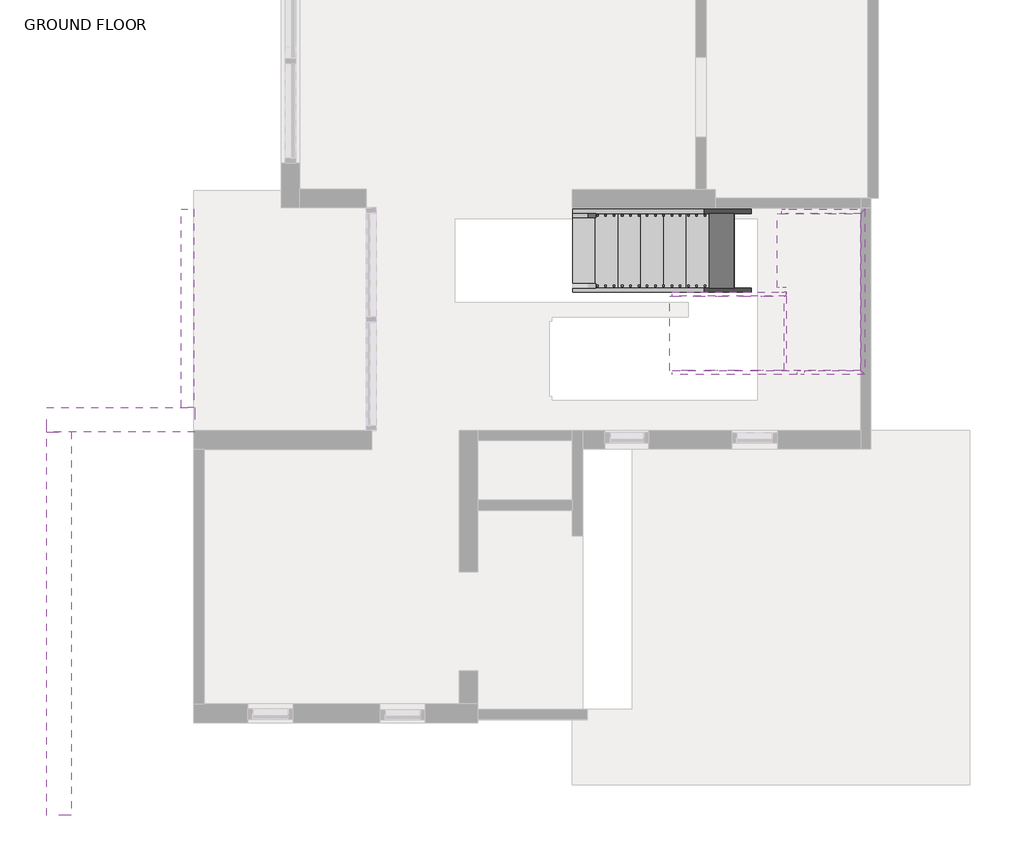
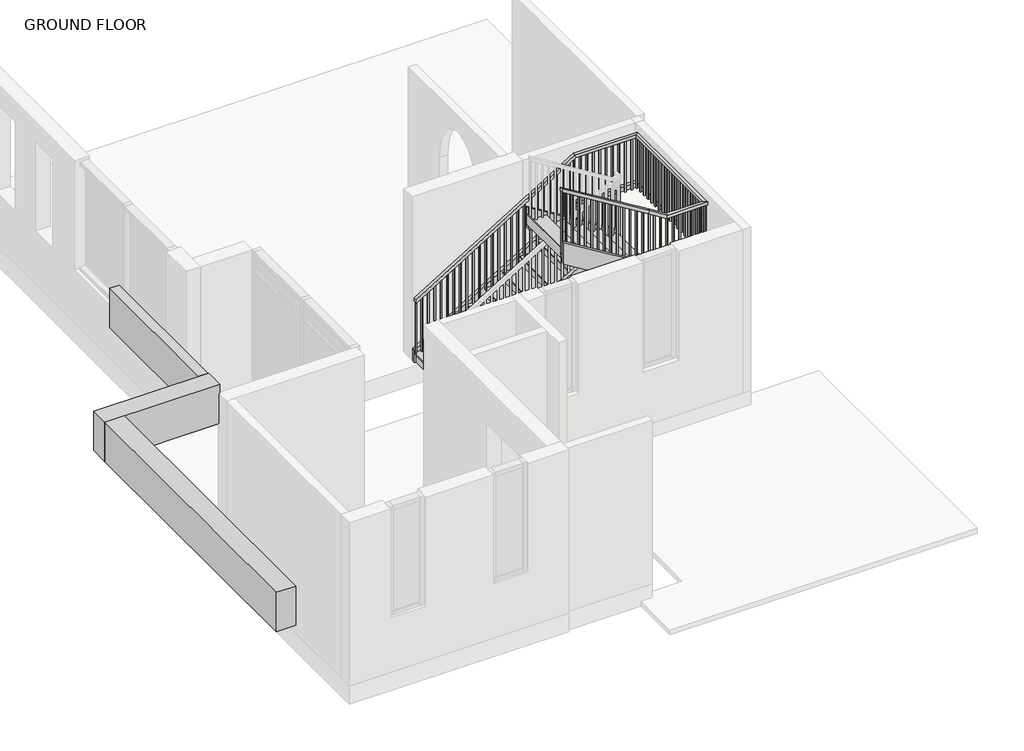
# One storey, part 3 of 3: 8 members, 3 proxies, 2 stair flights, 1 railing, 1 slab.
"""IFC4 building model written with IfcOpenShell, lengths in millimetres."""

from ifc_helpers import new_model, si_unit, frame, origin, place, context, project, spatial, polyline, outline, extrude, faceted_brep, transform, mapped, element, save
from components import generic_models_11_generic_models_11_40482c90, generic_models_7_generic_models_7_1309f326, generic_models_8_generic_models_8_410e38da, non_monolithic_landing_593ffa06, stair_flight_f1cb69c7, stair_flight_ba00a610

model = new_model("IFC4")

# Units and contexts
model_context = context("Model", 3, world=origin())
ifc_project = project(units=[si_unit("LENGTHUNIT", "METRE", prefix="MILLI")], contexts=[model_context])

# Site, building, storey
site = spatial("IfcSite", under=ifc_project)
building = spatial("IfcBuilding", under=site)
storey = spatial("IfcBuildingStorey", under=building, Name="GROUND FLOOR", Elevation=304.8)

# Proxies
placement = place(None, origin())
generic_models_11_generic_models_11_shape = generic_models_11_generic_models_11_40482c90(model_context)
element("IfcBuildingElementProxy", 1, Name="Generic Models 11 : Generic Models 11", ObjectType="Generic Models 11 : Generic Models 11", at=placement, inside=storey, context=model_context, shape_type="MappedRepresentation", body=[
    mapped(generic_models_11_generic_models_11_shape, transform((0.0, 0.0, 0.0), x_axis=(1.0, 0.0, 0.0), y_axis=(0.0, 1.0, 0.0), z_axis=(0.0, 0.0, 1.0))),
])
generic_models_7_generic_models_7_shape = generic_models_7_generic_models_7_1309f326(model_context)
element("IfcBuildingElementProxy", 2, Name="Generic Models 7 : Generic Models 7", ObjectType="Generic Models 7 : Generic Models 7", at=placement, inside=storey, context=model_context, shape_type="MappedRepresentation", body=[
    mapped(generic_models_7_generic_models_7_shape, transform((0.0, 0.0, 0.0), x_axis=(1.0, 0.0, 0.0), y_axis=(0.0, 1.0, 0.0), z_axis=(0.0, 0.0, 1.0))),
])
generic_models_8_generic_models_8_shape = generic_models_8_generic_models_8_410e38da(model_context)
element("IfcBuildingElementProxy", 3, Name="Generic Models 8 : Generic Models 8", ObjectType="Generic Models 8 : Generic Models 8", at=placement, inside=storey, context=model_context, shape_type="MappedRepresentation", body=[
    mapped(generic_models_8_generic_models_8_shape, transform((0.0, 0.0, 0.0), x_axis=(1.0, 0.0, 0.0), y_axis=(0.0, 1.0, 0.0), z_axis=(0.0, 0.0, 1.0))),
])

# Members
element("IfcMember", 4, ObjectType="Stringer - 2\" Width", at=placement, inside=storey, context=model_context, shape_type="SweptSolid", body=[
    extrude(outline(polyline([(517.6257693, -8269.5911408), (304.8, -8269.5911408), (304.8, -8033.644807), (1790.7, -5612.1781404), (2095.5, -5698.2405426), (517.6257693, -8269.5911408)])), frame((0.0, -5310.3337491, 0.0), z_axis=(0.0, 1.0, 0.0), x_axis=(0.0, 0.0, 1.0)), (0.0, 0.0, 1.0), 50.8),
])
element("IfcMember", 5, ObjectType="Stringer - 2\" Width", at=placement, inside=storey, context=model_context, shape_type="SweptSolid", body=[
    extrude(outline(polyline([(517.6257693, -8269.5911408), (304.8, -8269.5911408), (304.8, -8033.644807), (1769.0092306, -5647.5260609), (2095.5, -5647.5260609), (2095.5, -5698.2405426), (517.6257693, -8269.5911408)])), frame((0.0, -6275.5337491, 0.0), z_axis=(0.0, 1.0, 0.0), x_axis=(0.0, 0.0, 1.0)), (0.0, 0.0, 1.0), 50.8),
])
element("IfcMember", 6, ObjectType="Stringer - 2\" Width", at=placement, inside=storey, context=model_context, shape_type="SweptSolid", body=[
    extrude(outline(polyline([(1790.7, -5510.9390614), (2095.5, -5424.8766591), (3089.3757693, -7044.5260609), (2731.7647497, -7044.5260609), (1790.7, -5510.9390614)])), frame((0.0, -7293.1310793, 0.0), z_axis=(0.0, 1.0, 0.0), x_axis=(0.0, 0.0, 1.0)), (0.0, 0.0, 1.0), 50.8),
])
element("IfcMember", 7, ObjectType="Stringer - 2\" Width", at=placement, inside=storey, context=model_context, shape_type="SweptSolid", body=[
    extrude(outline(polyline([(1874.5147497, -5647.5260609), (2232.1257693, -5647.5260609), (3089.3757693, -7044.5260609), (2731.7647497, -7044.5260609), (1874.5147497, -5647.5260609)])), frame((0.0, -6327.9310793, 0.0), z_axis=(0.0, 1.0, 0.0), x_axis=(0.0, 0.0, 1.0)), (0.0, 0.0, 1.0), 50.8),
])
element("IfcMember", 8, ObjectType="Stringer - 2\" Width", at=placement, inside=storey, context=model_context, shape_type="Brep", body=[
    faceted_brep([(-5424.8766591, -7242.3310793, 2095.5), (-5424.8766591, -7293.1310793, 2095.5), (-4682.3260609, -7293.1310793, 2095.5), (-4733.1260609, -7242.3310793, 2095.5), (-5510.9390614, -7242.3310793, 1790.7), (-4733.1260609, -7242.3310793, 1790.7), (-5510.9390614, -7293.1310793, 1790.7), (-4682.3260609, -7293.1310793, 1790.7)], [[[0, 1, 2, 3]], [[4, 0, 3, 5]], [[6, 4, 5, 7]], [[1, 6, 7, 2]], [[1, 0, 4, 6]], [[2, 7, 5, 3]]]),
])
element("IfcMember", 9, ObjectType="Stringer - 2\" Width", at=placement, inside=storey, context=model_context, shape_type="SweptSolid", body=[
    extrude(outline(polyline([(-4682.3260609, -7293.1310793), (-4733.1260609, -7242.3310793), (-4733.1260609, -5310.3337491), (-4682.3260609, -5259.5337491), (-4682.3260609, -7293.1310793)])), frame((0.0, 0.0, 1790.7), z_axis=(0.0, 0.0, 1.0), x_axis=(1.0, 0.0, 0.0)), (0.0, 0.0, 1.0), 304.8),
])
element("IfcMember", 10, ObjectType="Stringer - 2\" Width", at=placement, inside=storey, context=model_context, shape_type="Brep", body=[
    faceted_brep([(-4733.1260609, -5310.3337491, 2095.5), (-4682.3260609, -5259.5337491, 2095.5), (-5698.2405426, -5259.5337491, 2095.5), (-5698.2405426, -5310.3337491, 2095.5), (-4733.1260609, -5310.3337491, 1790.7), (-5612.1781404, -5310.3337491, 1790.7), (-4682.3260609, -5259.5337491, 1790.7), (-5612.1781404, -5259.5337491, 1790.7)], [[[0, 1, 2, 3]], [[4, 0, 3, 5]], [[6, 4, 5, 7]], [[1, 6, 7, 2]], [[1, 0, 4, 6]], [[2, 7, 5, 3]]]),
])
element("IfcMember", 11, ObjectType="Stringer - 2\" Width", at=placement, inside=storey, context=model_context, shape_type="SweptSolid", body=[
    extrude(outline(polyline([(-5698.3260609, -6275.5337491), (-5647.5260609, -6275.5337491), (-5647.5260609, -6277.1310793), (-5698.3260609, -6277.1310793), (-5698.3260609, -6275.5337491)])), frame((0.0, 0.0, 1790.7), z_axis=(0.0, 0.0, 1.0), x_axis=(1.0, 0.0, 0.0)), (0.0, 0.0, 1.0), 304.8),
])

# Railing
element("IfcRailing", 12, ObjectType="Handrail - Rectangular", at=placement, inside=storey, context=model_context, shape_type="SolidModel", body=[
    faceted_brep([(-8269.5911408, -5310.3337491, 1390.65), (-8269.5911408, -5310.3337491, 1331.0481634), (-8269.5911408, -5361.1337491, 1331.0481634), (-8269.5911408, -5361.1337491, 1390.65), (-5754.9911408, -5310.3337491, 2933.7), (-5740.6474071, -5310.3337491, 2882.9), (-5740.6474071, -5361.1337491, 2882.9), (-5754.9911408, -5361.1337491, 2933.7), (-4733.1260609, -5310.3337491, 2933.7), (-4733.1260609, -5310.3337491, 2882.9), (-4783.9260609, -5361.1337491, 2882.9), (-4783.9260609, -5361.1337491, 2933.7), (-4733.1260609, -7242.3310793, 2933.7), (-4733.1260609, -7242.3310793, 2882.9), (-4783.9260609, -7191.5310793, 2882.9), (-4783.9260609, -7191.5310793, 2933.7), (-5368.1260609, -7242.3310793, 2933.7), (-5382.4697946, -7242.3310793, 2882.9), (-5382.4697946, -7191.5310793, 2882.9), (-5368.1260609, -7191.5310793, 2933.7), (-5647.5260609, -7242.3310793, 3105.15), (-5674.0952849, -7242.3310793, 3061.8520054), (-5674.0952849, -7191.5310793, 3061.8520054), (-5647.5260609, -7191.5310793, 3105.15), (-7044.5260609, -7242.3310793, 3962.4), (-7044.5260609, -7191.5310793, 3962.4), (-7044.5260609, -7191.5310793, 3902.7981634), (-7044.5260609, -7242.3310793, 3902.7981634)], [[[0, 1, 2, 3]], [[1, 0, 4, 5]], [[2, 1, 5, 6]], [[3, 2, 6, 7]], [[0, 3, 7, 4]], [[5, 4, 8, 9]], [[6, 5, 9, 10]], [[7, 6, 10, 11]], [[4, 7, 11, 8]], [[9, 8, 12, 13]], [[10, 9, 13, 14]], [[11, 10, 14, 15]], [[8, 11, 15, 12]], [[13, 12, 16, 17]], [[14, 13, 17, 18]], [[15, 14, 18, 19]], [[12, 15, 19, 16]], [[17, 16, 20, 21]], [[18, 17, 21, 22]], [[19, 18, 22, 23]], [[16, 19, 23, 20]], [[24, 25, 26, 27]], [[21, 20, 24, 27]], [[22, 21, 27, 26]], [[23, 22, 26, 25]], [[20, 23, 25, 24]]]),
    extrude(outline(polyline([(3861.8839589, -6977.8510609), (2876.55, -6977.8510609), (2876.55, -6958.8010609), (3850.1941861, -6958.8010609), (3861.8839589, -6977.8510609)])), frame((0.0, -7226.4560793, 0.0), z_axis=(0.0, 1.0, 0.0), x_axis=(0.0, 0.0, 1.0)), (0.0, 0.0, 1.0), 19.05),
    extrude(outline(polyline([(3799.5385043, -6876.2510609), (2876.55, -6876.2510609), (2876.55, -6857.2010609), (3787.8487316, -6857.2010609), (3799.5385043, -6876.2510609)])), frame((0.0, -7226.4560793, 0.0), z_axis=(0.0, 1.0, 0.0), x_axis=(0.0, 0.0, 1.0)), (0.0, 0.0, 1.0), 19.05),
    extrude(outline(polyline([(3737.1930498, -6774.6510609), (2876.55, -6774.6510609), (2876.55, -6755.6010609), (3725.503277, -6755.6010609), (3737.1930498, -6774.6510609)])), frame((0.0, -7226.4560793, 0.0), z_axis=(0.0, 1.0, 0.0), x_axis=(0.0, 0.0, 1.0)), (0.0, 0.0, 1.0), 19.05),
    extrude(outline(polyline([(3674.8475952, -6673.0510609), (2705.1, -6673.0510609), (2705.1, -6654.0010609), (3663.1578225, -6654.0010609), (3674.8475952, -6673.0510609)])), frame((0.0, -7226.4560793, 0.0), z_axis=(0.0, 1.0, 0.0), x_axis=(0.0, 0.0, 1.0)), (0.0, 0.0, 1.0), 19.05),
    extrude(outline(polyline([(3612.5021407, -6571.4510609), (2705.1, -6571.4510609), (2705.1, -6552.4010609), (3600.8123679, -6552.4010609), (3612.5021407, -6571.4510609)])), frame((0.0, -7226.4560793, 0.0), z_axis=(0.0, 1.0, 0.0), x_axis=(0.0, 0.0, 1.0)), (0.0, 0.0, 1.0), 19.05),
    extrude(outline(polyline([(3550.1566861, -6469.8510609), (2533.65, -6469.8510609), (2533.65, -6450.8010609), (3538.4669134, -6450.8010609), (3550.1566861, -6469.8510609)])), frame((0.0, -7226.4560793, 0.0), z_axis=(0.0, 1.0, 0.0), x_axis=(0.0, 0.0, 1.0)), (0.0, 0.0, 1.0), 19.05),
    extrude(outline(polyline([(3487.8112316, -6368.2510609), (2533.65, -6368.2510609), (2533.65, -6349.2010609), (3476.1214589, -6349.2010609), (3487.8112316, -6368.2510609)])), frame((0.0, -7226.4560793, 0.0), z_axis=(0.0, 1.0, 0.0), x_axis=(0.0, 0.0, 1.0)), (0.0, 0.0, 1.0), 19.05),
    extrude(outline(polyline([(3425.465777, -6266.6510609), (2533.65, -6266.6510609), (2533.65, -6247.6010609), (3413.7760043, -6247.6010609), (3425.465777, -6266.6510609)])), frame((0.0, -7226.4560793, 0.0), z_axis=(0.0, 1.0, 0.0), x_axis=(0.0, 0.0, 1.0)), (0.0, 0.0, 1.0), 19.05),
    extrude(outline(polyline([(3363.1203225, -6165.0510609), (2362.2, -6165.0510609), (2362.2, -6146.0010609), (3351.4305498, -6146.0010609), (3363.1203225, -6165.0510609)])), frame((0.0, -7226.4560793, 0.0), z_axis=(0.0, 1.0, 0.0), x_axis=(0.0, 0.0, 1.0)), (0.0, 0.0, 1.0), 19.05),
    extrude(outline(polyline([(3300.7748679, -6063.4510609), (2362.2, -6063.4510609), (2362.2, -6044.4010609), (3289.0850952, -6044.4010609), (3300.7748679, -6063.4510609)])), frame((0.0, -7226.4560793, 0.0), z_axis=(0.0, 1.0, 0.0), x_axis=(0.0, 0.0, 1.0)), (0.0, 0.0, 1.0), 19.05),
    extrude(outline(polyline([(3238.4294134, -5961.8510609), (2362.2, -5961.8510609), (2362.2, -5942.8010609), (3226.7396407, -5942.8010609), (3238.4294134, -5961.8510609)])), frame((0.0, -7226.4560793, 0.0), z_axis=(0.0, 1.0, 0.0), x_axis=(0.0, 0.0, 1.0)), (0.0, 0.0, 1.0), 19.05),
    extrude(outline(polyline([(3176.0839589, -5860.2510609), (2190.75, -5860.2510609), (2190.75, -5841.2010609), (3164.3941861, -5841.2010609), (3176.0839589, -5860.2510609)])), frame((0.0, -7226.4560793, 0.0), z_axis=(0.0, 1.0, 0.0), x_axis=(0.0, 0.0, 1.0)), (0.0, 0.0, 1.0), 19.05),
    extrude(outline(polyline([(3113.7385043, -5758.6510609), (2190.75, -5758.6510609), (2190.75, -5739.6010609), (3102.0487316, -5739.6010609), (3113.7385043, -5758.6510609)])), frame((0.0, -7226.4560793, 0.0), z_axis=(0.0, 1.0, 0.0), x_axis=(0.0, 0.0, 1.0)), (0.0, 0.0, 1.0), 19.05),
    extrude(outline(polyline([(3004.6339589, -5580.8510609), (2019.3, -5580.8510609), (2019.3, -5561.8010609), (2992.9441861, -5561.8010609), (3004.6339589, -5580.8510609)])), frame((0.0, -7226.4560793, 0.0), z_axis=(0.0, 1.0, 0.0), x_axis=(0.0, 0.0, 1.0)), (0.0, 0.0, 1.0), 19.05),
    extrude(outline(polyline([(2942.2885043, -5479.2510609), (2019.3, -5479.2510609), (2019.3, -5460.2010609), (2930.5987316, -5460.2010609), (2942.2885043, -5479.2510609)])), frame((0.0, -7226.4560793, 0.0), z_axis=(0.0, 1.0, 0.0), x_axis=(0.0, 0.0, 1.0)), (0.0, 0.0, 1.0), 19.05),
    extrude(outline(polyline([(-5358.6010609, -7226.4560793), (-5377.6510609, -7226.4560793), (-5377.6510609, -7207.4060793), (-5358.6010609, -7207.4060793), (-5358.6010609, -7226.4560793)])), frame((0.0, 0.0, 2019.3), z_axis=(0.0, 0.0, 1.0), x_axis=(1.0, 0.0, 0.0)), (0.0, 0.0, 1.0), 863.6),
    extrude(outline(polyline([(-5257.0010609, -7226.4560793), (-5276.0510609, -7226.4560793), (-5276.0510609, -7207.4060793), (-5257.0010609, -7207.4060793), (-5257.0010609, -7226.4560793)])), frame((0.0, 0.0, 2019.3), z_axis=(0.0, 0.0, 1.0), x_axis=(1.0, 0.0, 0.0)), (0.0, 0.0, 1.0), 863.6),
    extrude(outline(polyline([(-5155.4010609, -7226.4560793), (-5174.4510609, -7226.4560793), (-5174.4510609, -7207.4060793), (-5155.4010609, -7207.4060793), (-5155.4010609, -7226.4560793)])), frame((0.0, 0.0, 2019.3), z_axis=(0.0, 0.0, 1.0), x_axis=(1.0, 0.0, 0.0)), (0.0, 0.0, 1.0), 863.6),
    extrude(outline(polyline([(-5053.8010609, -7226.4560793), (-5072.8510609, -7226.4560793), (-5072.8510609, -7207.4060793), (-5053.8010609, -7207.4060793), (-5053.8010609, -7226.4560793)])), frame((0.0, 0.0, 2019.3), z_axis=(0.0, 0.0, 1.0), x_axis=(1.0, 0.0, 0.0)), (0.0, 0.0, 1.0), 863.6),
    extrude(outline(polyline([(-4952.2010609, -7226.4560793), (-4971.2510609, -7226.4560793), (-4971.2510609, -7207.4060793), (-4952.2010609, -7207.4060793), (-4952.2010609, -7226.4560793)])), frame((0.0, 0.0, 2019.3), z_axis=(0.0, 0.0, 1.0), x_axis=(1.0, 0.0, 0.0)), (0.0, 0.0, 1.0), 863.6),
    extrude(outline(polyline([(-4850.6010609, -7226.4560793), (-4869.6510609, -7226.4560793), (-4869.6510609, -7207.4060793), (-4850.6010609, -7207.4060793), (-4850.6010609, -7226.4560793)])), frame((0.0, 0.0, 2019.3), z_axis=(0.0, 0.0, 1.0), x_axis=(1.0, 0.0, 0.0)), (0.0, 0.0, 1.0), 863.6),
    extrude(outline(polyline([(-4749.0010609, -7155.0087491), (-4749.0010609, -7174.0587491), (-4768.0510609, -7174.0587491), (-4768.0510609, -7155.0087491), (-4749.0010609, -7155.0087491)])), frame((0.0, 0.0, 2019.3), z_axis=(0.0, 0.0, 1.0), x_axis=(1.0, 0.0, 0.0)), (0.0, 0.0, 1.0), 863.6),
    extrude(outline(polyline([(-4749.0010609, -7053.4087491), (-4749.0010609, -7072.4587491), (-4768.0510609, -7072.4587491), (-4768.0510609, -7053.4087491), (-4749.0010609, -7053.4087491)])), frame((0.0, 0.0, 2019.3), z_axis=(0.0, 0.0, 1.0), x_axis=(1.0, 0.0, 0.0)), (0.0, 0.0, 1.0), 863.6),
    extrude(outline(polyline([(-4749.0010609, -6951.8087491), (-4749.0010609, -6970.8587491), (-4768.0510609, -6970.8587491), (-4768.0510609, -6951.8087491), (-4749.0010609, -6951.8087491)])), frame((0.0, 0.0, 2019.3), z_axis=(0.0, 0.0, 1.0), x_axis=(1.0, 0.0, 0.0)), (0.0, 0.0, 1.0), 863.6),
    extrude(outline(polyline([(-4749.0010609, -6850.2087491), (-4749.0010609, -6869.2587491), (-4768.0510609, -6869.2587491), (-4768.0510609, -6850.2087491), (-4749.0010609, -6850.2087491)])), frame((0.0, 0.0, 2019.3), z_axis=(0.0, 0.0, 1.0), x_axis=(1.0, 0.0, 0.0)), (0.0, 0.0, 1.0), 863.6),
    extrude(outline(polyline([(-4749.0010609, -6748.6087491), (-4749.0010609, -6767.6587491), (-4768.0510609, -6767.6587491), (-4768.0510609, -6748.6087491), (-4749.0010609, -6748.6087491)])), frame((0.0, 0.0, 2019.3), z_axis=(0.0, 0.0, 1.0), x_axis=(1.0, 0.0, 0.0)), (0.0, 0.0, 1.0), 863.6),
    extrude(outline(polyline([(-4749.0010609, -6647.0087491), (-4749.0010609, -6666.0587491), (-4768.0510609, -6666.0587491), (-4768.0510609, -6647.0087491), (-4749.0010609, -6647.0087491)])), frame((0.0, 0.0, 2019.3), z_axis=(0.0, 0.0, 1.0), x_axis=(1.0, 0.0, 0.0)), (0.0, 0.0, 1.0), 863.6),
    extrude(outline(polyline([(-4749.0010609, -6545.4087491), (-4749.0010609, -6564.4587491), (-4768.0510609, -6564.4587491), (-4768.0510609, -6545.4087491), (-4749.0010609, -6545.4087491)])), frame((0.0, 0.0, 2019.3), z_axis=(0.0, 0.0, 1.0), x_axis=(1.0, 0.0, 0.0)), (0.0, 0.0, 1.0), 863.6),
    extrude(outline(polyline([(-4749.0010609, -6443.8087491), (-4749.0010609, -6462.8587491), (-4768.0510609, -6462.8587491), (-4768.0510609, -6443.8087491), (-4749.0010609, -6443.8087491)])), frame((0.0, 0.0, 2019.3), z_axis=(0.0, 0.0, 1.0), x_axis=(1.0, 0.0, 0.0)), (0.0, 0.0, 1.0), 863.6),
    extrude(outline(polyline([(-4749.0010609, -6342.2087491), (-4749.0010609, -6361.2587491), (-4768.0510609, -6361.2587491), (-4768.0510609, -6342.2087491), (-4749.0010609, -6342.2087491)])), frame((0.0, 0.0, 2019.3), z_axis=(0.0, 0.0, 1.0), x_axis=(1.0, 0.0, 0.0)), (0.0, 0.0, 1.0), 863.6),
    extrude(outline(polyline([(-4749.0010609, -6240.6087491), (-4749.0010609, -6259.6587491), (-4768.0510609, -6259.6587491), (-4768.0510609, -6240.6087491), (-4749.0010609, -6240.6087491)])), frame((0.0, 0.0, 2019.3), z_axis=(0.0, 0.0, 1.0), x_axis=(1.0, 0.0, 0.0)), (0.0, 0.0, 1.0), 863.6),
    extrude(outline(polyline([(-4749.0010609, -6139.0087491), (-4749.0010609, -6158.0587491), (-4768.0510609, -6158.0587491), (-4768.0510609, -6139.0087491), (-4749.0010609, -6139.0087491)])), frame((0.0, 0.0, 2019.3), z_axis=(0.0, 0.0, 1.0), x_axis=(1.0, 0.0, 0.0)), (0.0, 0.0, 1.0), 863.6),
    extrude(outline(polyline([(-4749.0010609, -6037.4087491), (-4749.0010609, -6056.4587491), (-4768.0510609, -6056.4587491), (-4768.0510609, -6037.4087491), (-4749.0010609, -6037.4087491)])), frame((0.0, 0.0, 2019.3), z_axis=(0.0, 0.0, 1.0), x_axis=(1.0, 0.0, 0.0)), (0.0, 0.0, 1.0), 863.6),
    extrude(outline(polyline([(-4749.0010609, -5935.8087491), (-4749.0010609, -5954.8587491), (-4768.0510609, -5954.8587491), (-4768.0510609, -5935.8087491), (-4749.0010609, -5935.8087491)])), frame((0.0, 0.0, 2019.3), z_axis=(0.0, 0.0, 1.0), x_axis=(1.0, 0.0, 0.0)), (0.0, 0.0, 1.0), 863.6),
    extrude(outline(polyline([(-4749.0010609, -5834.2087491), (-4749.0010609, -5853.2587491), (-4768.0510609, -5853.2587491), (-4768.0510609, -5834.2087491), (-4749.0010609, -5834.2087491)])), frame((0.0, 0.0, 2019.3), z_axis=(0.0, 0.0, 1.0), x_axis=(1.0, 0.0, 0.0)), (0.0, 0.0, 1.0), 863.6),
    extrude(outline(polyline([(-4749.0010609, -5732.6087491), (-4749.0010609, -5751.6587491), (-4768.0510609, -5751.6587491), (-4768.0510609, -5732.6087491), (-4749.0010609, -5732.6087491)])), frame((0.0, 0.0, 2019.3), z_axis=(0.0, 0.0, 1.0), x_axis=(1.0, 0.0, 0.0)), (0.0, 0.0, 1.0), 863.6),
    extrude(outline(polyline([(-4749.0010609, -5631.0087491), (-4749.0010609, -5650.0587491), (-4768.0510609, -5650.0587491), (-4768.0510609, -5631.0087491), (-4749.0010609, -5631.0087491)])), frame((0.0, 0.0, 2019.3), z_axis=(0.0, 0.0, 1.0), x_axis=(1.0, 0.0, 0.0)), (0.0, 0.0, 1.0), 863.6),
    extrude(outline(polyline([(-4749.0010609, -5529.4087491), (-4749.0010609, -5548.4587491), (-4768.0510609, -5548.4587491), (-4768.0510609, -5529.4087491), (-4749.0010609, -5529.4087491)])), frame((0.0, 0.0, 2019.3), z_axis=(0.0, 0.0, 1.0), x_axis=(1.0, 0.0, 0.0)), (0.0, 0.0, 1.0), 863.6),
    extrude(outline(polyline([(-4749.0010609, -5427.8087491), (-4749.0010609, -5446.8587491), (-4768.0510609, -5446.8587491), (-4768.0510609, -5427.8087491), (-4749.0010609, -5427.8087491)])), frame((0.0, 0.0, 2019.3), z_axis=(0.0, 0.0, 1.0), x_axis=(1.0, 0.0, 0.0)), (0.0, 0.0, 1.0), 863.6),
    extrude(outline(polyline([(-4850.1161408, -5326.2087491), (-4831.0661408, -5326.2087491), (-4831.0661408, -5345.2587491), (-4850.1161408, -5345.2587491), (-4850.1161408, -5326.2087491)])), frame((0.0, 0.0, 2019.3), z_axis=(0.0, 0.0, 1.0), x_axis=(1.0, 0.0, 0.0)), (0.0, 0.0, 1.0), 863.6),
    extrude(outline(polyline([(-4951.7161408, -5326.2087491), (-4932.6661408, -5326.2087491), (-4932.6661408, -5345.2587491), (-4951.7161408, -5345.2587491), (-4951.7161408, -5326.2087491)])), frame((0.0, 0.0, 2019.3), z_axis=(0.0, 0.0, 1.0), x_axis=(1.0, 0.0, 0.0)), (0.0, 0.0, 1.0), 863.6),
    extrude(outline(polyline([(-5053.3161408, -5326.2087491), (-5034.2661408, -5326.2087491), (-5034.2661408, -5345.2587491), (-5053.3161408, -5345.2587491), (-5053.3161408, -5326.2087491)])), frame((0.0, 0.0, 2019.3), z_axis=(0.0, 0.0, 1.0), x_axis=(1.0, 0.0, 0.0)), (0.0, 0.0, 1.0), 863.6),
    extrude(outline(polyline([(-5154.9161408, -5326.2087491), (-5135.8661408, -5326.2087491), (-5135.8661408, -5345.2587491), (-5154.9161408, -5345.2587491), (-5154.9161408, -5326.2087491)])), frame((0.0, 0.0, 2019.3), z_axis=(0.0, 0.0, 1.0), x_axis=(1.0, 0.0, 0.0)), (0.0, 0.0, 1.0), 863.6),
    extrude(outline(polyline([(-5256.5161408, -5326.2087491), (-5237.4661408, -5326.2087491), (-5237.4661408, -5345.2587491), (-5256.5161408, -5345.2587491), (-5256.5161408, -5326.2087491)])), frame((0.0, 0.0, 2019.3), z_axis=(0.0, 0.0, 1.0), x_axis=(1.0, 0.0, 0.0)), (0.0, 0.0, 1.0), 863.6),
    extrude(outline(polyline([(-5358.1161408, -5326.2087491), (-5339.0661408, -5326.2087491), (-5339.0661408, -5345.2587491), (-5358.1161408, -5345.2587491), (-5358.1161408, -5326.2087491)])), frame((0.0, 0.0, 2019.3), z_axis=(0.0, 0.0, 1.0), x_axis=(1.0, 0.0, 0.0)), (0.0, 0.0, 1.0), 863.6),
    extrude(outline(polyline([(-5459.7161408, -5326.2087491), (-5440.6661408, -5326.2087491), (-5440.6661408, -5345.2587491), (-5459.7161408, -5345.2587491), (-5459.7161408, -5326.2087491)])), frame((0.0, 0.0, 2019.3), z_axis=(0.0, 0.0, 1.0), x_axis=(1.0, 0.0, 0.0)), (0.0, 0.0, 1.0), 863.6),
    extrude(outline(polyline([(-5561.3161408, -5326.2087491), (-5542.2661408, -5326.2087491), (-5542.2661408, -5345.2587491), (-5561.3161408, -5345.2587491), (-5561.3161408, -5326.2087491)])), frame((0.0, 0.0, 2019.3), z_axis=(0.0, 0.0, 1.0), x_axis=(1.0, 0.0, 0.0)), (0.0, 0.0, 1.0), 863.6),
    extrude(outline(polyline([(-5662.9161408, -5326.2087491), (-5643.8661408, -5326.2087491), (-5643.8661408, -5345.2587491), (-5662.9161408, -5345.2587491), (-5662.9161408, -5326.2087491)])), frame((0.0, 0.0, 2019.3), z_axis=(0.0, 0.0, 1.0), x_axis=(1.0, 0.0, 0.0)), (0.0, 0.0, 1.0), 863.6),
    extrude(outline(polyline([(2821.4941861, -5840.7161408), (1847.85, -5840.7161408), (1847.85, -5821.6661408), (2833.1839589, -5821.6661408), (2821.4941861, -5840.7161408)])), frame((0.0, -5345.2587491, 0.0), z_axis=(0.0, 1.0, 0.0), x_axis=(0.0, 0.0, 1.0)), (0.0, 0.0, 1.0), 19.05),
    extrude(outline(polyline([(2759.1487316, -5942.3161408), (1847.85, -5942.3161408), (1847.85, -5923.2661408), (2770.8385043, -5923.2661408), (2759.1487316, -5942.3161408)])), frame((0.0, -5345.2587491, 0.0), z_axis=(0.0, 1.0, 0.0), x_axis=(0.0, 0.0, 1.0)), (0.0, 0.0, 1.0), 19.05),
    extrude(outline(polyline([(2696.803277, -6043.9161408), (1847.85, -6043.9161408), (1847.85, -6024.8661408), (2708.4930498, -6024.8661408), (2696.803277, -6043.9161408)])), frame((0.0, -5345.2587491, 0.0), z_axis=(0.0, 1.0, 0.0), x_axis=(0.0, 0.0, 1.0)), (0.0, 0.0, 1.0), 19.05),
    extrude(outline(polyline([(2634.4578225, -6145.5161408), (1676.4, -6145.5161408), (1676.4, -6126.4661408), (2646.1475952, -6126.4661408), (2634.4578225, -6145.5161408)])), frame((0.0, -5345.2587491, 0.0), z_axis=(0.0, 1.0, 0.0), x_axis=(0.0, 0.0, 1.0)), (0.0, 0.0, 1.0), 19.05),
    extrude(outline(polyline([(2572.1123679, -6247.1161408), (1676.4, -6247.1161408), (1676.4, -6228.0661408), (2583.8021407, -6228.0661408), (2572.1123679, -6247.1161408)])), frame((0.0, -5345.2587491, 0.0), z_axis=(0.0, 1.0, 0.0), x_axis=(0.0, 0.0, 1.0)), (0.0, 0.0, 1.0), 19.05),
    extrude(outline(polyline([(2509.7669134, -6348.7161408), (1504.95, -6348.7161408), (1504.95, -6329.6661408), (2521.4566861, -6329.6661408), (2509.7669134, -6348.7161408)])), frame((0.0, -5345.2587491, 0.0), z_axis=(0.0, 1.0, 0.0), x_axis=(0.0, 0.0, 1.0)), (0.0, 0.0, 1.0), 19.05),
    extrude(outline(polyline([(2447.4214589, -6450.3161408), (1504.95, -6450.3161408), (1504.95, -6431.2661408), (2459.1112316, -6431.2661408), (2447.4214589, -6450.3161408)])), frame((0.0, -5345.2587491, 0.0), z_axis=(0.0, 1.0, 0.0), x_axis=(0.0, 0.0, 1.0)), (0.0, 0.0, 1.0), 19.05),
    extrude(outline(polyline([(2385.0760043, -6551.9161408), (1504.95, -6551.9161408), (1504.95, -6532.8661408), (2396.765777, -6532.8661408), (2385.0760043, -6551.9161408)])), frame((0.0, -5345.2587491, 0.0), z_axis=(0.0, 1.0, 0.0), x_axis=(0.0, 0.0, 1.0)), (0.0, 0.0, 1.0), 19.05),
    extrude(outline(polyline([(2322.7305498, -6653.5161408), (1333.5, -6653.5161408), (1333.5, -6634.4661408), (2334.4203225, -6634.4661408), (2322.7305498, -6653.5161408)])), frame((0.0, -5345.2587491, 0.0), z_axis=(0.0, 1.0, 0.0), x_axis=(0.0, 0.0, 1.0)), (0.0, 0.0, 1.0), 19.05),
    extrude(outline(polyline([(2260.3850952, -6755.1161408), (1333.5, -6755.1161408), (1333.5, -6736.0661408), (2272.0748679, -6736.0661408), (2260.3850952, -6755.1161408)])), frame((0.0, -5345.2587491, 0.0), z_axis=(0.0, 1.0, 0.0), x_axis=(0.0, 0.0, 1.0)), (0.0, 0.0, 1.0), 19.05),
    extrude(outline(polyline([(2198.0396407, -6856.7161408), (1333.5, -6856.7161408), (1333.5, -6837.6661408), (2209.7294134, -6837.6661408), (2198.0396407, -6856.7161408)])), frame((0.0, -5345.2587491, 0.0), z_axis=(0.0, 1.0, 0.0), x_axis=(0.0, 0.0, 1.0)), (0.0, 0.0, 1.0), 19.05),
    extrude(outline(polyline([(2135.6941861, -6958.3161408), (1162.05, -6958.3161408), (1162.05, -6939.2661408), (2147.3839589, -6939.2661408), (2135.6941861, -6958.3161408)])), frame((0.0, -5345.2587491, 0.0), z_axis=(0.0, 1.0, 0.0), x_axis=(0.0, 0.0, 1.0)), (0.0, 0.0, 1.0), 19.05),
    extrude(outline(polyline([(2073.3487316, -7059.9161408), (1162.05, -7059.9161408), (1162.05, -7040.8661408), (2085.0385043, -7040.8661408), (2073.3487316, -7059.9161408)])), frame((0.0, -5345.2587491, 0.0), z_axis=(0.0, 1.0, 0.0), x_axis=(0.0, 0.0, 1.0)), (0.0, 0.0, 1.0), 19.05),
    extrude(outline(polyline([(2011.003277, -7161.5161408), (1162.05, -7161.5161408), (1162.05, -7142.4661408), (2022.6930498, -7142.4661408), (2011.003277, -7161.5161408)])), frame((0.0, -5345.2587491, 0.0), z_axis=(0.0, 1.0, 0.0), x_axis=(0.0, 0.0, 1.0)), (0.0, 0.0, 1.0), 19.05),
    extrude(outline(polyline([(1948.6578225, -7263.1161408), (990.6, -7263.1161408), (990.6, -7244.0661408), (1960.3475952, -7244.0661408), (1948.6578225, -7263.1161408)])), frame((0.0, -5345.2587491, 0.0), z_axis=(0.0, 1.0, 0.0), x_axis=(0.0, 0.0, 1.0)), (0.0, 0.0, 1.0), 19.05),
    extrude(outline(polyline([(1886.3123679, -7364.7161408), (990.6, -7364.7161408), (990.6, -7345.6661408), (1898.0021407, -7345.6661408), (1886.3123679, -7364.7161408)])), frame((0.0, -5345.2587491, 0.0), z_axis=(0.0, 1.0, 0.0), x_axis=(0.0, 0.0, 1.0)), (0.0, 0.0, 1.0), 19.05),
    extrude(outline(polyline([(1823.9669134, -7466.3161408), (819.15, -7466.3161408), (819.15, -7447.2661408), (1835.6566861, -7447.2661408), (1823.9669134, -7466.3161408)])), frame((0.0, -5345.2587491, 0.0), z_axis=(0.0, 1.0, 0.0), x_axis=(0.0, 0.0, 1.0)), (0.0, 0.0, 1.0), 19.05),
    extrude(outline(polyline([(1761.6214589, -7567.9161408), (819.15, -7567.9161408), (819.15, -7548.8661408), (1773.3112316, -7548.8661408), (1761.6214589, -7567.9161408)])), frame((0.0, -5345.2587491, 0.0), z_axis=(0.0, 1.0, 0.0), x_axis=(0.0, 0.0, 1.0)), (0.0, 0.0, 1.0), 19.05),
    extrude(outline(polyline([(1699.2760043, -7669.5161408), (819.15, -7669.5161408), (819.15, -7650.4661408), (1710.965777, -7650.4661408), (1699.2760043, -7669.5161408)])), frame((0.0, -5345.2587491, 0.0), z_axis=(0.0, 1.0, 0.0), x_axis=(0.0, 0.0, 1.0)), (0.0, 0.0, 1.0), 19.05),
    extrude(outline(polyline([(1636.9305498, -7771.1161408), (647.7, -7771.1161408), (647.7, -7752.0661408), (1648.6203225, -7752.0661408), (1636.9305498, -7771.1161408)])), frame((0.0, -5345.2587491, 0.0), z_axis=(0.0, 1.0, 0.0), x_axis=(0.0, 0.0, 1.0)), (0.0, 0.0, 1.0), 19.05),
    extrude(outline(polyline([(1574.5850952, -7872.7161408), (647.7, -7872.7161408), (647.7, -7853.6661408), (1586.2748679, -7853.6661408), (1574.5850952, -7872.7161408)])), frame((0.0, -5345.2587491, 0.0), z_axis=(0.0, 1.0, 0.0), x_axis=(0.0, 0.0, 1.0)), (0.0, 0.0, 1.0), 19.05),
    extrude(outline(polyline([(1512.2396407, -7974.3161408), (647.7, -7974.3161408), (647.7, -7955.2661408), (1523.9294134, -7955.2661408), (1512.2396407, -7974.3161408)])), frame((0.0, -5345.2587491, 0.0), z_axis=(0.0, 1.0, 0.0), x_axis=(0.0, 0.0, 1.0)), (0.0, 0.0, 1.0), 19.05),
    extrude(outline(polyline([(1449.8941861, -8075.9161408), (476.25, -8075.9161408), (476.25, -8056.8661408), (1461.5839589, -8056.8661408), (1449.8941861, -8075.9161408)])), frame((0.0, -5345.2587491, 0.0), z_axis=(0.0, 1.0, 0.0), x_axis=(0.0, 0.0, 1.0)), (0.0, 0.0, 1.0), 19.05),
    extrude(outline(polyline([(1387.5487316, -8177.5161408), (476.25, -8177.5161408), (476.25, -8158.4661408), (1399.2385043, -8158.4661408), (1387.5487316, -8177.5161408)])), frame((0.0, -5345.2587491, 0.0), z_axis=(0.0, 1.0, 0.0), x_axis=(0.0, 0.0, 1.0)), (0.0, 0.0, 1.0), 19.05),
    extrude(outline(polyline([(3051.3930498, -5657.0510609), (2019.3, -5657.0510609), (2019.3, -5638.0010609), (3039.703277, -5638.0010609), (3051.3930498, -5657.0510609)])), frame((0.0, -7226.4560793, 0.0), z_axis=(0.0, 1.0, 0.0), x_axis=(0.0, 0.0, 1.0)), (0.0, 0.0, 1.0), 19.05),
    extrude(outline(polyline([(-4749.0010609, -7207.4060793), (-4749.0010609, -7226.4560793), (-4768.0510609, -7226.4560793), (-4768.0510609, -7207.4060793), (-4749.0010609, -7207.4060793)])), frame((0.0, 0.0, 2019.3), z_axis=(0.0, 0.0, 1.0), x_axis=(1.0, 0.0, 0.0)), (0.0, 0.0, 1.0), 863.6),
    extrude(outline(polyline([(-4768.0510609, -5326.2087491), (-4749.0010609, -5326.2087491), (-4749.0010609, -5345.2587491), (-4768.0510609, -5345.2587491), (-4768.0510609, -5326.2087491)])), frame((0.0, 0.0, 2019.3), z_axis=(0.0, 0.0, 1.0), x_axis=(1.0, 0.0, 0.0)), (0.0, 0.0, 1.0), 863.6),
    extrude(outline(polyline([(2868.253277, -5764.5161408), (2019.3, -5764.5161408), (2019.3, -5745.4661408), (2879.9430498, -5745.4661408), (2868.253277, -5764.5161408)])), frame((0.0, -5345.2587491, 0.0), z_axis=(0.0, 1.0, 0.0), x_axis=(0.0, 0.0, 1.0)), (0.0, 0.0, 1.0), 19.05),
    extrude(outline(polyline([(3902.7981634, -7044.5260609), (2876.55, -7044.5260609), (2876.55, -7025.4760609), (3891.1083907, -7025.4760609), (3902.7981634, -7044.5260609)])), frame((0.0, -7226.4560793, 0.0), z_axis=(0.0, 1.0, 0.0), x_axis=(0.0, 0.0, 1.0)), (0.0, 0.0, 1.0), 19.05),
    extrude(outline(polyline([(1331.0481634, -8269.5911408), (476.25, -8269.5911408), (476.25, -8250.5411408), (1342.7379361, -8250.5411408), (1331.0481634, -8269.5911408)])), frame((0.0, -5345.2587491, 0.0), z_axis=(0.0, 1.0, 0.0), x_axis=(0.0, 0.0, 1.0)), (0.0, 0.0, 1.0), 19.05),
])

# Slab
non_monolithic_landing_shape = non_monolithic_landing_593ffa06(model_context)
element("IfcSlab", 13, ObjectType="Non-Monolithic Landing", at=placement, inside=storey, context=model_context, shape_type="MappedRepresentation", body=[
    mapped(non_monolithic_landing_shape, transform((0.0, 0.0, 0.0), x_axis=(1.0, 0.0, 0.0), y_axis=(0.0, 1.0, 0.0), z_axis=(0.0, 0.0, 1.0))),
])

# Stair flights
stair_flight_shape = stair_flight_f1cb69c7(model_context)
element("IfcStairFlight", 14, ObjectType="2\" Tread 1\" Nosing 1/4\" Riser", at=placement, inside=storey, context=model_context, shape_type="MappedRepresentation", body=[
    mapped(stair_flight_shape, transform((0.0, 0.0, 0.0), x_axis=(1.0, 0.0, 0.0), y_axis=(0.0, 1.0, 0.0), z_axis=(0.0, 0.0, 1.0))),
])
stair_flight_2_shape = stair_flight_ba00a610(model_context)
element("IfcStairFlight", 15, ObjectType="2\" Tread 1\" Nosing 1/4\" Riser", at=placement, inside=storey, context=model_context, shape_type="MappedRepresentation", body=[
    mapped(stair_flight_2_shape, transform((0.0, 0.0, 0.0), x_axis=(1.0, 0.0, 0.0), y_axis=(0.0, 1.0, 0.0), z_axis=(0.0, 0.0, 1.0))),
])

save(model, "model.ifc")

# Revit data of these elements
# Type "Handrail - Rectangular"
#   Assembly Code = "C2010400"
#   built-in parameter 1008612 = 0.0416667 (stored number, unit not read)
#   built-in parameter 1008611 = 0.0416667 (stored number, unit not read)
#   built-in parameter 1008609 = 0.333333 (stored number, unit not read)
#   built-in parameter 1008604 = 0.166667 (stored number, unit not read)
#   built-in parameter 1008603 = 0.166667 (stored number, unit not read)
#   Railing Height = 3' - 0"
#   built-in parameter 1008630 = 2
#   built-in parameter 1008610 = 2
#   built-in parameter 1008618 = Baluster - Square : 3/4"
# Element 1 (IfcBuildingElementProxy, "Generic Models 11 : Generic Models 11")
#   Phase Created = New Construction
#   Materials on its faces: "GREY COLOUR FRAME(2)"
# Element 2 (IfcBuildingElementProxy, "Generic Models 7 : Generic Models 7")
#   Phase Created = New Construction
#   Materials on its faces: "GREY COLOUR FRAME(2)"
# Element 3 (IfcBuildingElementProxy, "Generic Models 8 : Generic Models 8")
#   Phase Created = New Construction
#   Materials on its faces: "GREY COLOUR FRAME(2)"
# Elements 4, 5, 6, 7, 8, 9, 10, 11 (IfcMember, "Stringer - 2\" Width")
#   Phase Created = New Construction
# Element 12 (IfcRailing, "Handrail - Rectangular")
#   Phase Created = New Construction
# Element 13 (IfcSlab, "Non-Monolithic Landing")
#   Phase Created = New Construction
# Elements 14, 15 (IfcStairFlight, "2\" Tread 1\" Nosing 1/4\" Riser")
#   Phase Created = New Construction
# Materials
#   "GREY COLOUR FRAME(2)": class "Generic", colour RGB 120 120 120, transparency 0, Cost = 0
